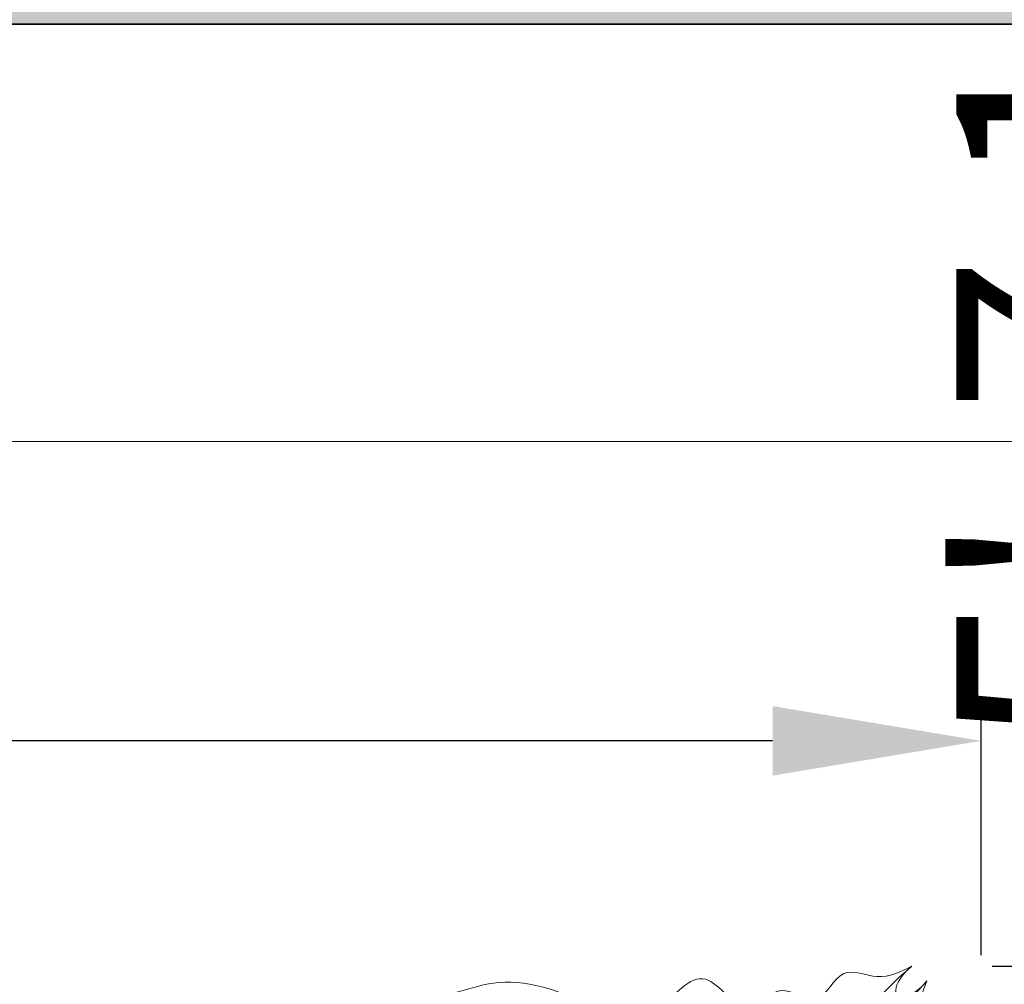
# Model space of a CAD drawing. Units: inches. Extents: x 2083 to 3317, y 1141 to 2115.
# Tile 13 of 256: x 2267 to 2324, y 1361 to 1417. Entities that reach past the tile are written whole.
import ezdxf

# ---------------------------------------------------------------- set-up
doc = ezdxf.new("R2010")
doc.units = ezdxf.units.IN
for name, color, linetype, lineweight in [('A-ANNO-DIMS', 2, 'Continuous', 18), ('A-FLOR-CASE', 8, 'Continuous', 18), ('A-FURN', 8, 'Continuous', 18), ('A-WALL', 7, 'Continuous', 35), ('www.cadblocksfree.com', 7, 'Continuous', 9)]:
    doc.layers.add(name, color=color, linetype=linetype, lineweight=lineweight)
doc.layers.add('A-WALL-PATT', color=251, linetype='Continuous', lineweight=13, true_color=0x636466)
doc.styles.get("Standard").update_dxf_attribs({"font": 'arial.ttf'})
doc.dimstyles.new('ISO-25', dxfattribs={"dimtxt": 12, "dimasz": 12, "dimexe": 1.25, "dimexo": 0.625, "dimtad": 1, "dimlunit": 3, "dimtxsty": 'Standard', "dimcen": 2.5, "dimadec": 0, "dimazin": 0, "dimtfac": 1, "dimtmove": 0, "dimatfit": 3, "dimfxl": 1, "dimarcsym": 0})

# ---------------------------------------------------------------- blocks, each defined once
blk = doc.blocks.new('bed')
at = {"layer": 'www.cadblocksfree.com', "ltscale": 0.2}
for centre, major_axis, ratio, start_param, end_param in [((3429.422, 1388.371), (-3.043, 3.043), 0.168252, 4.250342, 8.316029), ((3430.477, 1387.316), (-1.055, 1.055), 0.453532, 4.422107, 8.144264)]:
    blk.add_ellipse(centre, major_axis=major_axis, ratio=ratio, start_param=start_param, end_param=end_param, dxfattribs=at)
for points, knots in [([(3428.534, 1423.97), (3428.914, 1423.397), (3430.098, 1421.613), (3428.491, 1417.656), (3430.593, 1413.794), (3429.801, 1409.122), (3428.396, 1406.564), (3427.355, 1404.971)], [0, 0, 0, 0, 0.050513, 0.157399, 0.2842023, 0.3628173, 0.5066917, 0.5066917, 0.5066917, 0.5066917]), ([(3431.237, 1387.473), (3430.882, 1388.172), (3430.205, 1389.505), (3431.478, 1391.985), (3428.294, 1393.194), (3430.501, 1395.689), (3427.558, 1397.866), (3431.841, 1400.386), (3426.535, 1404.33), (3426.443, 1408.152), (3426.379, 1410.814)], [0, 0, 0, 0, 2.267059, 4.324559, 6.685584, 8.878641, 11.121502, 14.300359, 17.755284, 25.682856, 25.682856, 25.682856, 25.682856]), ([(3430.32, 1386.556), (3427.327, 1387.653), (3422.148, 1389.55), (3414.529, 1384.137), (3405.607, 1387.046), (3396.29, 1386.314), (3386.838, 1381.282), (3377.742, 1390.272), (3370.778, 1384.799), (3364.626, 1383.966), (3363.275, 1388.265), (3360.778, 1387.151), (3359.446, 1386.556)], [0, 0, 0, 0, 8.93042, 15.449194, 25.485629, 34.878505, 43.598887, 54.554403, 64.16647, 67.461673, 70.610457, 74.213583, 74.213583, 74.213583, 74.213583])]:
    blk.add_open_spline(points, degree=3, knots=knots, dxfattribs=at)
blk = doc.blocks.new('CASEWORK-96X24')
for q in [(0, 0), (24, 96)]:
    blk.add_line((0, 96), q)
blk = doc.blocks.new('*D22')
at = {"layer": 'A-ANNO-DIMS', "color": 0, "lineweight": -2, "transparency": 16777216}
for p, q in [((2235.96, 1362.739), (2235.96, 1376.309)), ((2322.26, 1362.739), (2322.26, 1376.309)), ((2235.96, 1375.059), (2083.007, 1375.059)), ((2310.26, 1375.059), (2247.96, 1375.059))]:
    blk.add_line(p, q, dxfattribs=at)
at = {"layer": 'A-ANNO-DIMS', "color": 0, "transparency": 16777216}
for points in [[(2247.96, 1377.059), (2247.96, 1373.059), (2235.96, 1375.059)], [(2310.26, 1377.059), (2310.26, 1373.059), (2322.26, 1375.059)]]:
    blk.add_solid(points, dxfattribs=at)
at = {"layer": 'Defpoints', "color": 0, "transparency": 16777216}
for p in [(2235.96, 1375.059), (2235.96, 1362.114), (2322.26, 1362.114)]:
    blk.add_point(p, dxfattribs=at)
at = {"layer": 'A-ANNO-DIMS', "color": 0, "transparency": 16777216, "insert": (2153.483, 1381.889), "char_height": 12, "attachment_point": 5}
blk.add_mtext('BED 7\'-2 1/2" TYP.', dxfattribs=at)
blk = doc.blocks.new('*D23')
at = {"layer": 'A-ANNO-DIMS', "color": 0, "lineweight": -2, "transparency": 16777216}
for p, q in [((2335.205, 1362.114), (2335.205, 1476.472)), ((2322.885, 1362.114), (2336.455, 1362.114)), ((2335.205, 1306.473), (2335.205, 1350.114)), ((2322.885, 1294.473), (2336.455, 1294.473))]:
    blk.add_line(p, q, dxfattribs=at)
at = {"layer": 'A-ANNO-DIMS', "color": 0, "transparency": 16777216}
for points in [[(2333.205, 1350.114), (2337.205, 1350.114), (2335.205, 1362.114)], [(2333.205, 1306.473), (2337.205, 1306.473), (2335.205, 1294.473)]]:
    blk.add_solid(points, dxfattribs=at)
at = {"layer": 'Defpoints', "color": 0, "transparency": 16777216}
for p in [(2322.26, 1362.114), (2335.205, 1362.114), (2322.26, 1294.473)]:
    blk.add_point(p, dxfattribs=at)
at = {"layer": 'A-ANNO-DIMS', "color": 0, "transparency": 16777216, "insert": (2328.376, 1425.293), "char_height": 12, "attachment_point": 5, "rotation": 90}
blk.add_mtext('5\'-7 1/2" TYP.', dxfattribs=at)
blk = doc.blocks.new('*D30')
at = {"layer": 'A-ANNO-DIMS', "color": 0, "lineweight": -2, "transparency": 16777216}
for p, q in [((2240.018, 1445.274), (2240.018, 1448.046)), ((2254.329, 1445.274), (2254.329, 1448.046)), ((2228.018, 1446.796), (2216.018, 1446.796)), ((2240.018, 1446.796), (2254.329, 1446.796)), ((2266.329, 1446.796), (2413.765, 1446.796))]:
    blk.add_line(p, q, dxfattribs=at)
at = {"layer": 'A-ANNO-DIMS', "color": 0, "transparency": 16777216}
for points in [[(2228.018, 1448.796), (2228.018, 1444.796), (2240.018, 1446.796)], [(2266.329, 1448.796), (2266.329, 1444.796), (2254.329, 1446.796)]]:
    blk.add_solid(points, dxfattribs=at)
at = {"layer": 'Defpoints', "color": 0, "transparency": 16777216}
for p in [(2254.329, 1446.796), (2240.018, 1444.649), (2254.329, 1444.649)]:
    blk.add_point(p, dxfattribs=at)
at = {"layer": 'A-ANNO-DIMS', "color": 0, "transparency": 16777216, "insert": (2346.047, 1453.625), "char_height": 12, "attachment_point": 5}
blk.add_mtext('WC 1\'-2 1/2" TYP.', dxfattribs=at)

msp = doc.modelspace()

# ---------------------------------------------------------------- hatches: boundary and pattern name
at = {"layer": 'A-WALL-PATT'}
h = msp.add_hatch(color=256, dxfattribs=at)
h.dxf.hatch_style = 1
h.paths.add_polyline_path([(3126.96, 2020.761), (2748.96, 2020.761), (2604.96, 2020.761), (2226.96, 2020.761), (2226.96, 1702.761), (2466.96, 1702.761), (2466.96, 1582.761), (2418.96, 1582.761), (2418.96, 1477.761), (2226.96, 1477.761), (2226.96, 1263.261), (2544.96, 1263.261), (2544.96, 1411.761), (2604.96, 1411.761), (2685.96, 1411.761), (2685.96, 1420.761), (2604.96, 1420.761), (2604.96, 1573.761), (2604.96, 1702.761), (2604.96, 2011.761), (2748.96, 2011.761), (2748.96, 1702.761), (2862.96, 1702.761), (2862.96, 1621.761), (2871.96, 1621.761), (2871.96, 1702.761), (2883.96, 1702.761), (2883.96, 1706.939, -0.026459), (2883.96, 1711.761), (2757.96, 1711.761), (2757.96, 1807.761), (2787.96, 1807.761), (2787.96, 1812.261), (2757.96, 1812.261), (2757.96, 2011.761), (2877.96, 2011.761), (2877.96, 1812.261), (2847.96, 1812.261), (2847.96, 1807.761), (2889.836, 1807.761), (2889.836, 1812.261), (2882.46, 1812.261), (2882.46, 2011.761), (3117.96, 2011.761), (3117.96, 1812.261), (2937.836, 1812.261), (2937.836, 1807.761), (2995.71, 1807.761), (2995.71, 1796.118), (3000.21, 1796.118), (3000.21, 1807.761), (3117.96, 1807.761), (3117.96, 1711.761), (3000.21, 1711.761), (3000.21, 1760.118), (2998.573, 1760.118, -0.020711), (2995.71, 1760.118), (2995.71, 1711.761), (2931.96, 1711.761), (2931.96, 1702.761), (3126.96, 1702.761)])
h.paths.add_polyline_path([(2471.46, 2011.761), (2471.46, 1810.011), (2462.717, 1810.011), (2462.717, 1805.511), (2505.96, 1805.511), (2505.96, 1810.011), (2475.96, 1810.011), (2475.96, 2011.761), (2595.96, 2011.761), (2595.96, 1810.011), (2565.96, 1810.011), (2565.96, 1805.511), (2595.96, 1805.511), (2595.96, 1711.761), (2235.96, 1711.761), (2235.96, 1805.511), (2353.71, 1805.511), (2353.71, 1796.054), (2358.21, 1796.054), (2358.21, 1805.511), (2414.717, 1805.511), (2414.717, 1810.011), (2235.96, 1810.011), (2235.96, 2011.761)], flags=16)
h.paths.add_polyline_path([(2270.205, 1994.61), (2270.205, 1970.61), (2246.205, 1970.61), (2246.205, 1994.61)], flags=0)
edge = h.paths.add_edge_path(flags=0)
edge.add_ellipse((2332.027, 1899.798), major_axis=(-3.043, 3.043), ratio=0.168252, start_angle=-161.3322, end_angle=-156.3071, ccw=False)
edge.add_ellipse((2333.082, 1898.744), major_axis=(-1.055, 1.055), ratio=0.453532, start_angle=-123.371, end_angle=-94.1591)
edge = h.paths.add_edge_path(flags=0)
edge.add_ellipse((2332.027, 1968.876), major_axis=(3.043, 3.043), ratio=0.168252, start_angle=18.6678, end_angle=23.6929)
edge.add_spline(control_points=[(2332.926, 1970.691), (2332.227, 1970.336), (2330.894, 1969.659), (2328.413, 1970.932), (2327.204, 1967.749), (2324.71, 1969.956), (2322.533, 1967.012), (2320.013, 1971.296), (2317.68, 1968.158), (2316.041, 1967.102), (2315.427, 1966.81)], knot_values=[0, 0, 0, 0, 2.267059, 4.324559, 6.685584, 8.878641, 11.121502, 14.300359, 17.755284, 19.732645, 19.732645, 19.732645, 19.732645], degree=3, periodic=0)
edge.add_ellipse((2332.027, 1968.876), major_axis=(3.043, 3.043), ratio=0.168252, start_angle=18.6678, end_angle=23.6929, ccw=False)
edge.add_ellipse((2333.082, 1969.931), major_axis=(1.055, 1.055), ratio=0.453532, start_angle=56.629, end_angle=85.8409, ccw=False)
edge = h.paths.add_edge_path(flags=0)
edge.add_spline(control_points=[(2296.428, 1967.988), (2293.628, 1965.336), (2287.704, 1959.727), (2299.744, 1949.996), (2294.533, 1935.669), (2290.573, 1920.604), (2293.394, 1909.974), (2296.185, 1904.967)], knot_values=[0.099185, 0.099185, 0.099185, 0.099185, 0.345301, 0.619822, 0.982653, 1.386093, 1.810555, 1.810555, 1.810555, 1.810555], degree=3, periodic=0)
edge.add_spline(control_points=[(2296.185, 1904.967), (2297.384, 1902.619), (2298.001, 1901.949), (2298.553, 1901.468)], knot_values=[0.006246, 0.006246, 0.006246, 0.006246, 0.055476, 0.055476, 0.055476, 0.055476], degree=3, periodic=0)
edge.add_spline(control_points=[(2298.553, 1901.468), (2297.259, 1900.923), (2295.225, 1900.232), (2293.06, 1900.614), (2292.101, 1900.788), (2292.09, 1900.791)], knot_values=[0.312835, 0.312835, 0.312835, 0.312835, 0.40178, 0.474987, 0.475903, 0.475903, 0.475903, 0.475903], degree=3, periodic=0)
edge.add_arc((2292.794, 1904.664), 3.937, 215.4209, 259.6982, ccw=False)
edge.add_spline(control_points=[(2289.585, 1902.382), (2289.477, 1902.535), (2289.368, 1902.688), (2289.261, 1902.841)], knot_values=[0.102872, 0.102872, 0.102872, 0.102872, 0.116896, 0.116896, 0.116896, 0.116896], degree=3, periodic=0)
edge.add_spline(control_points=[(2289.261, 1902.841), (2288.687, 1902.55), (2287.64, 1902.02), (2285.881, 1901.874), (2283.853, 1901.504), (2281.72, 1899.711), (2278.467, 1899.493), (2276.157, 1901.883), (2272.259, 1899.804), (2267.778, 1901.843), (2262.244, 1900.184), (2257.415, 1901.782), (2254.318, 1900.726), (2253.178, 1900.337)], knot_values=[0, 0, 0, 0, 1.907977, 3.477176, 5.261074, 7.972851, 11.680248, 13.717921, 16.939592, 22.789562, 27.502503, 33.595215, 37.145618, 37.145618, 37.145618, 37.145618], degree=3, periodic=0)
edge.add_line((2253.178, 1900.337), (2250.244, 1902.841))
edge.add_line((2250.244, 1902.841), (2250.244, 1965.833))
edge.add_line((2250.244, 1965.833), (2253.178, 1968.337))
edge.add_spline(control_points=[(2253.178, 1968.337), (2254.318, 1967.948), (2257.415, 1966.892), (2262.244, 1968.49), (2267.778, 1966.831), (2271.527, 1968.537), (2273.876, 1967.828), (2274.207, 1967.728)], knot_values=[0, 0, 0, 0, 0.09018, 0.244935, 0.364644, 0.513233, 0.537855, 0.537855, 0.537855, 0.537855], degree=3, periodic=0)
edge.add_arc((2274.353, 1963.793), 3.937, 72.0511, 92.1279, ccw=False)
edge.add_arc((2281.297, 1985.23), 18.596, 252.0511, 288.5657)
edge.add_arc((2292.317, 1956.029), 12.646, 71.0268, 113.7782, ccw=False)
edge = h.paths.add_edge_path(flags=0)
edge.add_spline(control_points=[(2274.899, 1951.856), (2275.066, 1951.617), (2275.233, 1951.377), (2275.398, 1951.136)], knot_values=[1.409916, 1.409916, 1.409916, 1.409916, 1.43159, 1.43159, 1.43159, 1.43159], degree=3, periodic=0)
edge.add_spline(control_points=[(2275.398, 1951.136), (2275.792, 1950.562), (2276.179, 1949.984), (2276.546, 1949.397)], knot_values=[1.358238, 1.358238, 1.358238, 1.358238, 1.409916, 1.409916, 1.409916, 1.409916], degree=3, periodic=0)
edge.add_line((2276.546, 1949.397), (2277.437, 1947.862))
edge.add_spline(control_points=[(2277.437, 1947.862), (2276.304, 1945.673), (2274.64, 1942.427), (2274.632, 1938.094), (2272.799, 1930.852), (2274.356, 1943.897), (2275.948, 1947.923), (2276.546, 1949.397)], knot_values=[0.005632, 0.005632, 0.005632, 0.005632, 0.186014, 0.266002, 0.357087, 0.59639, 0.739732, 0.739732, 0.739732, 0.739732], degree=3, periodic=0)
edge.add_spline(control_points=[(2276.546, 1949.397), (2276.179, 1949.984), (2275.792, 1950.562), (2275.398, 1951.136)], knot_values=[1.358238, 1.358238, 1.358238, 1.358238, 1.409916, 1.409916, 1.409916, 1.409916], degree=3, periodic=0)
edge.add_spline(control_points=[(2275.398, 1951.136), (2274.943, 1950.08), (2274.208, 1948.025), (2273.935, 1944.851), (2272.469, 1937.627), (2273.466, 1945.696), (2274.701, 1951.059), (2274.899, 1951.856)], knot_values=[0.104364, 0.104364, 0.104364, 0.104364, 0.189636, 0.269624, 0.36071, 0.600013, 0.644622, 0.644622, 0.644622, 0.644622], degree=3, periodic=0)
h.paths.add_polyline_path([(2269.168, 1963.128, -0.357527), (2268.171, 1960.976, -0.092561), (2268.171, 1939.436, -0.357527), (2269.168, 1937.285, -0.357527), (2267.016, 1938.282, -0.164785), (2254.686, 1938.282, -0.357527), (2252.534, 1937.285, -0.357527), (2253.531, 1939.436, -0.092561), (2253.531, 1960.976, -0.357527), (2252.534, 1963.128, -0.357527), (2254.686, 1962.131, -0.164785), (2267.016, 1962.131, -0.357527)], flags=0)
h.paths.add_polyline_path([(2248.874, 1967.802), (2248.874, 1957.028), (2249.458, 1957.028), (2249.458, 1911.647), (2248.874, 1911.647), (2248.874, 1900.873), (2246.512, 1900.873, 0.197327), (2244.15, 1902.457), (2244.15, 1966.218, 0.197327), (2246.512, 1967.802)], flags=0)
h.paths.add_polyline_path([(2269.168, 1931.389, -0.357527), (2268.171, 1929.238, -0.092561), (2268.171, 1907.698, -0.357527), (2269.168, 1905.547, -0.357527), (2267.016, 1906.544, -0.164785), (2254.686, 1906.544, -0.357527), (2252.534, 1905.547, -0.357527), (2253.531, 1907.698, -0.092561), (2253.531, 1929.238, -0.357527), (2252.534, 1931.389, -0.357527), (2254.686, 1930.392, -0.164785), (2267.016, 1930.392, -0.357527)], flags=0)
edge = h.paths.add_edge_path(flags=0)
edge.add_spline(control_points=[(2276.197, 1906.724), (2276.168, 1909.029), (2276.114, 1913.372), (2270.598, 1924.925), (2273.905, 1919.013), (2275.922, 1916.262), (2275.475, 1912.402), (2277.258, 1910.381), (2276.696, 1908.225), (2276.646, 1906.813), (2276.618, 1906.008)], knot_values=[0, 0, 0, 0, 8.61026, 16.221274, 18.843057, 23.804898, 27.440828, 29.356102, 31.203478, 33.650687, 33.650687, 33.650687, 33.650687], degree=3, periodic=0)
edge.add_spline(control_points=[(2276.618, 1906.008), (2276.623, 1905.624), (2276.498, 1904.629), (2275.442, 1903.855), (2274.937, 1903.08), (2274.859, 1902.841)], knot_values=[0.156488, 0.156488, 0.156488, 0.156488, 0.184398, 0.231376, 0.250598, 0.250598, 0.250598, 0.250598], degree=3, periodic=0)
edge.add_line((2274.859, 1902.841), (2276.506, 1902.841))
edge.add_spline(control_points=[(2276.506, 1902.841), (2276.788, 1903.085), (2277.665, 1904.125), (2278.25, 1904.341), (2277.654, 1908.527), (2278.156, 1906.228), (2278.1, 1905.286), (2278.847, 1904.069), (2277.857, 1903.415), (2277.874, 1902.991), (2277.904, 1902.841)], knot_values=[0.059574, 0.059574, 0.059574, 0.059574, 0.080753, 0.103741, 0.16972, 0.176036, 0.207137, 0.240474, 0.262341, 0.27366, 0.27366, 0.27366, 0.27366], degree=3, periodic=0)
edge.add_line((2277.904, 1902.841), (2280.03, 1902.841))
edge.add_spline(control_points=[(2280.03, 1902.841), (2279.888, 1903.088), (2279.499, 1903.982), (2280.152, 1905.939), (2278.104, 1909.658), (2279.762, 1907.185), (2280.328, 1904.875), (2280.485, 1903.49), (2281.463, 1903.249), (2281.758, 1902.936), (2281.834, 1902.841)], knot_values=[0.013856, 0.013856, 0.013856, 0.013856, 0.034874, 0.088867, 0.107879, 0.126738, 0.158714, 0.193757, 0.217487, 0.226722, 0.226722, 0.226722, 0.226722], degree=3, periodic=0)
edge.add_spline(control_points=[(2281.834, 1902.841), (2281.788, 1902.827), (2281.647, 1902.783), (2281.396, 1902.859), (2281.088, 1902.985), (2280.721, 1903.061), (2280.333, 1903.026), (2280.125, 1902.899), (2280.03, 1902.841)], knot_values=[0, 0, 0, 0, 0.14413, 0.435517, 0.749276, 1.153046, 1.548371, 1.878348, 1.878348, 1.878348, 1.878348], degree=3, periodic=0)
edge.add_line((2280.03, 1902.841), (2277.904, 1902.841))
edge.add_spline(control_points=[(2277.904, 1902.841), (2277.893, 1902.796), (2277.865, 1902.68), (2277.607, 1902.687), (2277.274, 1902.801), (2276.838, 1902.62), (2276.584, 1902.789), (2276.506, 1902.841)], knot_values=[0, 0, 0, 0, 0.127189, 0.326199, 0.628009, 1.24357, 1.515331, 1.515331, 1.515331, 1.515331], degree=3, periodic=0)
edge.add_line((2276.506, 1902.841), (2274.859, 1902.841))
edge.add_spline(control_points=[(2274.859, 1902.841), (2274.814, 1902.899), (2274.725, 1903.013), (2274.493, 1903.119), (2274.244, 1902.961), (2273.937, 1903.185), (2273.614, 1902.983), (2273.408, 1902.883), (2273.322, 1902.841)], knot_values=[0, 0, 0, 0, 0.21843, 0.436957, 0.687977, 0.990379, 1.398396, 1.69185, 1.69185, 1.69185, 1.69185], degree=3, periodic=0)
edge.add_spline(control_points=[(2273.322, 1902.841), (2273.617, 1903.446), (2274.274, 1904.538), (2276.027, 1904.574), (2276.207, 1906.584), (2276.197, 1906.724)], knot_values=[0.012227, 0.012227, 0.012227, 0.012227, 0.059472, 0.106218, 0.134458, 0.134458, 0.134458, 0.134458], degree=3, periodic=0)
h.paths.add_polyline_path([(2270.776, 1897.79), (2270.776, 1873.79), (2246.776, 1873.79), (2246.776, 1897.79)], flags=0)
h.paths.add_polyline_path([(2353.71, 1760.005), (2353.71, 1760.054), (2358.21, 1760.054, -0.033729)], flags=0)
h.paths.add_polyline_path([(2321.819, 1737.529), (2341.995, 1737.529, -0.414214), (2343.203, 1736.321), (2343.203, 1721.021, -0.414214), (2341.995, 1719.813), (2321.819, 1719.813, -0.414214), (2320.611, 1721.021), (2320.611, 1736.321, -0.414214)], flags=0)
h.paths.add_polyline_path([(2324.235, 1736.321), (2339.579, 1736.321, -0.414214), (2341.995, 1733.905), (2341.995, 1725.45, -0.414214), (2339.579, 1723.034), (2333.681, 1723.034), (2333.845, 1722.045, -0.870646), (2335.425, 1721.826, -0.767327), (2333.923, 1721.423), (2331.291, 1721.423, -0.767327), (2329.788, 1721.826, -0.870646), (2331.368, 1722.045), (2331.533, 1723.034), (2324.235, 1723.034, -0.414214), (2321.819, 1725.45), (2321.819, 1733.905, -0.414214)], flags=0)
h.paths.add_polyline_path([(2570.484, 1928.615), (2589.684, 1928.615), (2590.169, 1928.615), (2590.169, 1904.993), (2570.484, 1904.993)], flags=0)
h.paths.add_polyline_path([(2574.447, 1927.264, -1), (2572.829, 1927.264, -1)], flags=0)
h.paths.add_polyline_path([(2573.09, 1926.941), (2573.925, 1927.776), (2574.148, 1927.553), (2573.313, 1926.718)], flags=0)
h.paths.add_polyline_path([(2578.779, 1919.73, -1), (2571.592, 1919.73, -1)], flags=0)
h.paths.add_polyline_path([(2578.385, 1919.73, -1), (2571.985, 1919.73, -1)], flags=0)
h.paths.add_polyline_path([(2331.596, 1729.476, -1), (2333.618, 1729.476, -1)], flags=0)
h.paths.add_polyline_path([(2578.034, 1927.264, -1), (2576.416, 1927.264, -1)], flags=0)
h.paths.add_polyline_path([(2576.689, 1927.531), (2576.912, 1927.754), (2577.747, 1926.919), (2577.524, 1926.696)], flags=0)
h.paths.add_polyline_path([(2578.139, 1909.86, -1), (2572.232, 1909.86, -1)], flags=0)
h.paths.add_polyline_path([(2577.745, 1909.86, -1), (2572.625, 1909.86, -1)], flags=0)
h.paths.add_polyline_path([(2583.798, 1927.264, -1), (2582.179, 1927.264, -1)], flags=0)
h.paths.add_polyline_path([(2582.719, 1927.754), (2583.554, 1926.919), (2583.331, 1926.696), (2582.496, 1927.531)], flags=0)
h.paths.add_polyline_path([(2582.496, 1927.531), (2582.719, 1927.754), (2583.554, 1926.919), (2583.331, 1926.696)], flags=0)
h.paths.add_polyline_path([(2587.739, 1920.53, -1), (2581.832, 1920.53, -1)], flags=0)
h.paths.add_polyline_path([(2587.345, 1920.53, -1), (2582.225, 1920.53, -1)], flags=0)
h.paths.add_polyline_path([(2587.385, 1927.264, -1), (2585.766, 1927.264, -1)], flags=0)
h.paths.add_polyline_path([(2586.082, 1926.98), (2586.917, 1927.815), (2587.14, 1927.593), (2586.305, 1926.758)], flags=0)
h.paths.add_polyline_path([(2588.379, 1910.66, -1), (2581.192, 1910.66, -1)], flags=0)
h.paths.add_polyline_path([(2587.985, 1910.66, -1), (2581.585, 1910.66, -1)], flags=0)
h.paths.add_polyline_path([(2417.168, 1729.478), (2437.344, 1729.478, -0.414214), (2438.552, 1728.27), (2438.552, 1712.969, -0.414214), (2437.344, 1711.761), (2417.168, 1711.761, -0.414214), (2415.96, 1712.969), (2415.96, 1728.27, -0.414214)], flags=0)
h.paths.add_polyline_path([(2419.584, 1728.27), (2434.928, 1728.27, -0.414214), (2437.344, 1725.854), (2437.344, 1717.398, -0.414214), (2434.928, 1714.983), (2429.029, 1714.983), (2429.194, 1713.994, -0.870646), (2430.774, 1713.775, -0.767327), (2429.271, 1713.372), (2426.64, 1713.372, -0.767327), (2425.137, 1713.775, -0.870646), (2426.717, 1713.994), (2426.882, 1714.983), (2419.584, 1714.983, -0.414214), (2417.168, 1717.398), (2417.168, 1725.854, -0.414214)], flags=0)
h.paths.add_polyline_path([(2419.584, 1728.27), (2434.928, 1728.27, -0.414214), (2437.344, 1725.854), (2437.344, 1717.398, -0.414214), (2434.928, 1714.983), (2429.029, 1714.983), (2428.358, 1719.009), (2427.553, 1719.009), (2426.882, 1714.983), (2419.584, 1714.983, -0.414214), (2417.168, 1717.398), (2417.168, 1725.854, -0.414214)], flags=0)
h.paths.add_polyline_path([(2426.944, 1721.425, -1), (2428.967, 1721.425, -1)], flags=0)
h.paths.add_polyline_path([(2475.96, 1702.761), (2595.96, 1702.761), (2595.96, 1582.761), (2475.96, 1582.761)], flags=16)
h.paths.add_polyline_path([(2427.96, 1573.761), (2595.96, 1573.761), (2595.96, 1468.761), (2595.96, 1420.761), (2384.46, 1420.761), (2384.46, 1468.761), (2427.96, 1468.761)], flags=16)
h.paths.add_polyline_path([(2379.96, 1468.761), (2379.96, 1420.761), (2235.96, 1420.761), (2235.96, 1468.761)], flags=16)
h.paths.add_polyline_path([(2317.816, 1466.696), (2337.992, 1466.696, -0.414214), (2339.2, 1465.488), (2339.2, 1450.187, -0.414214), (2337.992, 1448.979), (2317.816, 1448.979, -0.414214), (2316.608, 1450.187), (2316.608, 1465.488, -0.414214)], flags=0)
h.paths.add_polyline_path([(2320.232, 1465.488), (2335.576, 1465.488, -0.414214), (2337.992, 1463.072), (2337.992, 1454.616, -0.414214), (2335.576, 1452.2), (2329.677, 1452.2), (2329.842, 1451.212, -0.870646), (2331.422, 1450.992, -0.767327), (2329.92, 1450.59), (2327.288, 1450.59, -0.767327), (2325.785, 1450.992, -0.870646), (2327.365, 1451.212), (2327.53, 1452.2), (2320.232, 1452.2, -0.414214), (2317.816, 1454.616), (2317.816, 1463.072, -0.414214)], flags=0)
h.paths.add_polyline_path([(2320.232, 1465.488), (2335.576, 1465.488, -0.414214), (2337.992, 1463.072), (2337.992, 1454.616, -0.414214), (2335.576, 1452.2), (2329.677, 1452.2), (2329.006, 1456.227), (2328.201, 1456.227), (2327.53, 1452.2), (2320.232, 1452.2, -0.414214), (2317.816, 1454.616), (2317.816, 1463.072, -0.414214)], flags=0)
h.paths.add_polyline_path([(2327.593, 1458.643, -1), (2329.615, 1458.643, -1)], flags=0)
h.paths.add_polyline_path([(2244.412, 1433.34), (2241.921, 1433.34, -0.414214), (2240.018, 1435.244), (2240.018, 1440.953, -0.414211), (2241.921, 1442.856), (2244.412, 1442.856, -1.976472)], flags=0)
h.paths.add_polyline_path([(2245.357, 1434.398, -0.414214), (2245.357, 1441.799, -2.144098)], flags=0)
h.paths.add_polyline_path([(2535.96, 1416.261), (2535.96, 1272.261), (2235.96, 1272.261), (2235.96, 1416.261)], flags=16)
h.paths.add_polyline_path([(2260.12, 1384.293), (2260.12, 1362.039), (2237.865, 1362.039), (2237.865, 1384.293)], flags=0)
edge = h.paths.add_edge_path(flags=0)
edge.add_line((2318.252, 1362.093), (2318.146, 1362.001))
edge.add_ellipse((2317.445, 1360.431), major_axis=(2.822, 2.822), ratio=0.168252, start_angle=18.6678, end_angle=20.9481, ccw=False)
edge.add_ellipse((2318.423, 1361.409), major_axis=(0.978, 0.978), ratio=0.453532, start_angle=56.629, end_angle=70.2262, ccw=False)
edge = h.paths.add_edge_path(flags=0)
edge.add_line((2319.107, 1295.571), (2319.015, 1295.677))
edge.add_ellipse((2317.445, 1296.378), major_axis=(-2.822, 2.822), ratio=0.168252, start_angle=-161.3322, end_angle=-159.0519, ccw=False)
edge.add_ellipse((2318.423, 1295.4), major_axis=(-0.978, 0.978), ratio=0.453532, start_angle=-123.371, end_angle=-109.7738)
edge = h.paths.add_edge_path(flags=0)
edge.add_spline(control_points=[(2284.21, 1301.17), (2284.581, 1300.445), (2284.891, 1299.892), (2285.16, 1299.461)], knot_values=[0.039066, 0.039066, 0.039066, 0.039066, 0.055476, 0.055476, 0.055476, 0.055476], degree=3, periodic=0)
edge.add_line((2285.16, 1299.461), (2284.21, 1301.17))
edge = h.paths.add_edge_path(flags=0)
edge.add_line((2280.412, 1297.298), (2283.37, 1297.036))
edge.add_line((2283.37, 1297.036), (2286.406, 1297.926))
edge.add_spline(control_points=[(2286.406, 1297.926), (2285.305, 1297.463), (2284.345, 1297.129), (2283.37, 1297.036)], knot_values=[0.394369, 0.394369, 0.394369, 0.394369, 0.475903, 0.475903, 0.475903, 0.475903], degree=3, periodic=0)
edge.add_spline(control_points=[(2283.37, 1297.036), (2283.281, 1297.028), (2282.316, 1296.957), (2281.313, 1297.134), (2280.423, 1297.296), (2280.412, 1297.298)], knot_values=[0.312835, 0.312835, 0.312835, 0.312835, 0.320246, 0.393453, 0.394369, 0.394369, 0.394369, 0.394369], degree=3, periodic=0)
edge = h.paths.add_edge_path(flags=0)
edge.add_line((2284.436, 1359.607), (2280.446, 1355.328))
edge.add_line((2280.446, 1355.328), (2279.58, 1351.018))
edge.add_line((2279.58, 1351.018), (2282.413, 1346.58))
edge.add_spline(control_points=[(2282.413, 1346.58), (2283.153, 1345.589), (2284.253, 1344.029), (2284.801, 1342.387), (2284.935, 1341.806)], knot_values=[1.240098, 1.240098, 1.240098, 1.240098, 1.332892, 1.382712, 1.382712, 1.382712, 1.382712], degree=3, periodic=0)
edge.add_spline(control_points=[(2284.935, 1341.806), (2285.319, 1340.141), (2285.233, 1338.409), (2284.91, 1336.654)], knot_values=[1.097484, 1.097484, 1.097484, 1.097484, 1.240098, 1.240098, 1.240098, 1.240098], degree=3, periodic=0)
edge.add_spline(control_points=[(2284.91, 1336.654), (2284.587, 1334.899), (2284.027, 1333.12), (2283.463, 1331.361)], knot_values=[0.95487, 0.95487, 0.95487, 0.95487, 1.097484, 1.097484, 1.097484, 1.097484], degree=3, periodic=0)
edge.add_line((2283.463, 1331.361), (2281.89, 1326.153))
edge.add_line((2281.89, 1326.153), (2280.756, 1321.056))
edge.add_line((2280.756, 1321.056), (2280.299, 1316.002))
edge.add_line((2280.299, 1316.002), (2280.716, 1310.95))
edge.add_line((2280.716, 1310.95), (2282.028, 1305.972))
edge.add_line((2282.028, 1305.972), (2284.21, 1301.17))
edge.add_spline(control_points=[(2284.21, 1301.17), (2283.341, 1302.73), (2282.612, 1304.336), (2282.028, 1305.972)], knot_values=[0.099185, 0.099185, 0.099185, 0.099185, 0.241799, 0.241799, 0.241799, 0.241799], degree=3, periodic=0)
edge.add_spline(control_points=[(2282.028, 1305.972), (2281.444, 1307.608), (2281.005, 1309.273), (2280.716, 1310.95)], knot_values=[0.241799, 0.241799, 0.241799, 0.241799, 0.384413, 0.384413, 0.384413, 0.384413], degree=3, periodic=0)
edge.add_spline(control_points=[(2280.716, 1310.95), (2280.433, 1312.588), (2280.289, 1314.277), (2280.299, 1315.962), (2280.299, 1316.002)], knot_values=[0.384413, 0.384413, 0.384413, 0.384413, 0.523647, 0.527028, 0.527028, 0.527028, 0.527028], degree=3, periodic=0)
edge.add_spline(control_points=[(2280.299, 1316.002), (2280.312, 1317.687), (2280.478, 1319.368), (2280.756, 1321.056)], knot_values=[0.527028, 0.527028, 0.527028, 0.527028, 0.669642, 0.669642, 0.669642, 0.669642], degree=3, periodic=0)
edge.add_spline(control_points=[(2280.756, 1321.056), (2281.035, 1322.744), (2281.426, 1324.44), (2281.89, 1326.153)], knot_values=[0.669642, 0.669642, 0.669642, 0.669642, 0.812256, 0.812256, 0.812256, 0.812256], degree=3, periodic=0)
edge.add_spline(control_points=[(2281.89, 1326.153), (2282.264, 1327.533), (2282.788, 1329.262), (2283.353, 1331.018), (2283.463, 1331.361)], knot_values=[0.812256, 0.812256, 0.812256, 0.812256, 0.927087, 0.95487, 0.95487, 0.95487, 0.95487], degree=3, periodic=0)
edge.add_line((2283.463, 1331.361), (2284.91, 1336.654))
edge.add_line((2284.91, 1336.654), (2284.935, 1341.806))
edge.add_line((2284.935, 1341.806), (2282.413, 1346.58))
edge.add_spline(control_points=[(2282.413, 1346.58), (2281.275, 1348.104), (2280.078, 1349.57), (2279.58, 1351.018)], knot_values=[1.382712, 1.382712, 1.382712, 1.382712, 1.525326, 1.525326, 1.525326, 1.525326], degree=3, periodic=0)
edge.add_spline(control_points=[(2279.58, 1351.018), (2279.443, 1351.415), (2279.136, 1352.857), (2279.735, 1354.29), (2280.446, 1355.328)], knot_values=[1.525326, 1.525326, 1.525326, 1.525326, 1.564439, 1.667941, 1.667941, 1.667941, 1.667941], degree=3, periodic=0)
edge.add_spline(control_points=[(2280.446, 1355.328), (2281.426, 1356.758), (2282.931, 1358.183), (2284.436, 1359.607)], knot_values=[1.667941, 1.667941, 1.667941, 1.667941, 1.810555, 1.810555, 1.810555, 1.810555], degree=3, periodic=0)
edge.add_arc((2280.623, 1348.518), 11.726, 71.0268, 113.7782)
edge.add_arc((2270.405, 1375.595), 17.244, 252.0511, 288.5657, ccw=False)
edge.add_arc((2263.966, 1355.718), 3.651, 72.0511, 92.1279)
edge.add_arc((2263.966, 1355.718), 3.651, 92.1279, 177.9851)
edge.add_spline(control_points=[(2260.318, 1355.846), (2260.26, 1354.221), (2260.551, 1350.187), (2262.999, 1346.766), (2264.473, 1344.649)], knot_values=[1.43159, 1.43159, 1.43159, 1.43159, 1.564144, 1.770695, 1.770695, 1.770695, 1.770695], degree=3, periodic=0)
edge.add_line((2264.473, 1344.649), (2264.936, 1343.983))
edge.add_spline(control_points=[(2263.801, 1340.248), (2263.843, 1340.514), (2264.067, 1341.756), (2264.513, 1343.002), (2264.935, 1343.981)], knot_values=[0.53657, 0.53657, 0.53657, 0.53657, 0.559349, 0.644622, 0.644622, 0.644622, 0.644622], degree=3, periodic=0)
edge.add_spline(control_points=[(2264.935, 1343.981), (2265.118, 1343.715), (2265.299, 1343.448), (2265.477, 1343.179)], knot_values=[1.384077, 1.384077, 1.384077, 1.384077, 1.409916, 1.409916, 1.409916, 1.409916], degree=3, periodic=0)
edge.add_spline(control_points=[(2265.477, 1343.179), (2265.655, 1342.911), (2265.829, 1342.641), (2265.999, 1342.369)], knot_values=[1.358238, 1.358238, 1.358238, 1.358238, 1.384077, 1.384077, 1.384077, 1.384077], degree=3, periodic=0)
edge.add_line((2265.999, 1342.369), (2266.826, 1340.946))
edge.add_spline(control_points=[(2266.826, 1340.946), (2268.894, 1337.09), (2271.398, 1325.843), (2270.516, 1310.569), (2275.919, 1301.861), (2277.79, 1299.199)], knot_values=[0.116896, 0.116896, 0.116896, 0.116896, 0.472987, 1.050969, 1.313793, 1.313793, 1.313793, 1.313793], degree=3, periodic=0)
edge.add_spline(control_points=[(2277.79, 1299.199), (2277.839, 1299.128), (2277.889, 1299.057), (2277.94, 1298.987)], knot_values=[0.109884, 0.109884, 0.109884, 0.109884, 0.116896, 0.116896, 0.116896, 0.116896], degree=3, periodic=0)
edge.add_line((2277.94, 1298.987), (2277.789, 1299.199))
edge.add_spline(control_points=[(2277.789, 1299.199), (2277.257, 1298.929), (2276.286, 1298.438), (2275.039, 1298.334), (2274.383, 1298.239), (2274.215, 1298.209)], knot_values=[33.12187, 33.12187, 33.12187, 33.12187, 35.029056, 36.598255, 37.144827, 37.144827, 37.144827, 37.144827], degree=3, periodic=0)
edge.add_line((2274.215, 1298.209), (2273.073, 1297.893))
edge.add_spline(control_points=[(2273.073, 1297.893), (2272.323, 1297.58), (2271.039, 1296.511), (2269.248, 1296.226), (2268.423, 1296.375)], knot_values=[26.532584, 26.532584, 26.532584, 26.532584, 29.198919, 31.839101, 31.839101, 31.839101, 31.839101], degree=3, periodic=0)
edge.add_line((2268.423, 1296.375), (2263.879, 1297.458))
edge.add_spline(control_points=[(2263.879, 1297.458), (2263.556, 1297.359), (2261.86, 1296.839), (2260.239, 1297.282), (2258.933, 1297.516)], knot_values=[15.919551, 15.919551, 15.919551, 15.919551, 16.939592, 21.226067, 21.226067, 21.226067, 21.226067], degree=3, periodic=0)
edge.add_line((2258.933, 1297.516), (2254.055, 1297.329))
edge.add_spline(control_points=[(2254.055, 1297.329), (2253.756, 1297.296), (2252.114, 1297.165), (2250.462, 1297.544), (2249.13, 1297.668)], knot_values=[5.306517, 5.306517, 5.306517, 5.306517, 6.276435, 10.613034, 10.613034, 10.613034, 10.613034], degree=3, periodic=0)
edge.add_line((2249.13, 1297.668), (2244.332, 1296.878))
edge.add_line((2244.332, 1296.878), (2241.611, 1299.199))
edge.add_line((2241.611, 1299.199), (2241.611, 1357.609))
edge.add_line((2241.611, 1357.609), (2244.332, 1359.931))
edge.add_line((2244.332, 1359.931), (2252.729, 1359.543))
edge.add_spline(control_points=[(2252.729, 1359.543), (2252.871, 1359.546), (2253.306, 1359.548), (2253.74, 1359.514), (2254.032, 1359.482)], knot_values=[0.233291, 0.233291, 0.233291, 0.233291, 0.244935, 0.268927, 0.268927, 0.268927, 0.268927], degree=3, periodic=0)
edge.add_line((2254.032, 1359.482), (2259.587, 1359.416))
edge.add_spline(control_points=[(2259.587, 1359.416), (2260.677, 1359.629), (2262.073, 1359.897), (2263.524, 1359.459), (2263.83, 1359.366)], knot_values=[0.422516, 0.422516, 0.422516, 0.422516, 0.513233, 0.537855, 0.537855, 0.537855, 0.537855], degree=3, periodic=0)
edge.add_arc((2263.966, 1355.718), 3.651, 72.0511, 92.1279, ccw=False)
edge.add_arc((2270.405, 1375.595), 17.244, 252.0511, 288.5657)
edge.add_arc((2280.623, 1348.518), 11.726, 71.0268, 113.7782, ccw=False)
h.paths.add_polyline_path([(2240.341, 1359.435), (2240.341, 1349.444), (2240.882, 1349.444), (2240.882, 1307.365), (2240.341, 1307.365), (2240.341, 1297.374), (2238.15, 1297.374, 0.197327), (2235.96, 1298.843), (2235.96, 1357.966, 0.197327), (2238.15, 1359.435)], flags=0)
h.paths.add_polyline_path([(2259.158, 1355.101, -0.357527), (2258.233, 1353.106, -0.092561), (2258.233, 1333.133, -0.357527), (2259.158, 1331.138, -0.357527), (2257.163, 1332.062, -0.164785), (2245.729, 1332.062, -0.357527), (2243.735, 1331.138, -0.357527), (2244.659, 1333.133, -0.092561), (2244.659, 1353.106, -0.357527), (2243.735, 1355.101, -0.357527), (2245.729, 1354.176, -0.164785), (2257.163, 1354.176, -0.357527)], flags=0)
edge = h.paths.add_edge_path(flags=0)
edge.add_line((2265.999, 1342.369), (2266.826, 1340.946))
edge.add_line((2266.826, 1340.946), (2265.308, 1337.814))
edge.add_line((2265.308, 1337.814), (2264.358, 1334.653))
edge.add_line((2264.358, 1334.653), (2264.262, 1333.8))
edge.add_spline(control_points=[(2264.262, 1333.8), (2264.208, 1333.187), (2264.162, 1332.366), (2264.007, 1331.414), (2263.969, 1331.202)], knot_values=[0.464444, 0.464444, 0.464444, 0.464444, 0.516691, 0.531608, 0.531608, 0.531608, 0.531608], degree=3, periodic=0)
edge.add_spline(control_points=[(2263.969, 1331.202), (2263.775, 1330.119), (2263.424, 1328.791), (2263.257, 1328.531), (2263.234, 1328.515)], knot_values=[0.372682, 0.372682, 0.372682, 0.372682, 0.44885, 0.464444, 0.464444, 0.464444, 0.464444], degree=3, periodic=0)
edge.add_spline(control_points=[(2263.234, 1328.515), (2263.096, 1328.42), (2263.131, 1329.301), (2263.275, 1330.616)], knot_values=[0.280919, 0.280919, 0.280919, 0.280919, 0.372682, 0.372682, 0.372682, 0.372682], degree=3, periodic=0)
edge.add_spline(control_points=[(2263.275, 1330.616), (2263.419, 1331.93), (2263.672, 1333.677), (2263.97, 1335.315)], knot_values=[0.189157, 0.189157, 0.189157, 0.189157, 0.280919, 0.280919, 0.280919, 0.280919], degree=3, periodic=0)
edge.add_spline(control_points=[(2263.97, 1335.315), (2264.1, 1336.032), (2264.419, 1337.622), (2264.755, 1338.864), (2264.947, 1339.491)], knot_values=[0.097394, 0.097394, 0.097394, 0.097394, 0.137578, 0.189157, 0.189157, 0.189157, 0.189157], degree=3, periodic=0)
edge.add_spline(control_points=[(2264.947, 1339.491), (2265.29, 1340.606), (2265.644, 1341.494), (2265.999, 1342.369)], knot_values=[0.005632, 0.005632, 0.005632, 0.005632, 0.097394, 0.097394, 0.097394, 0.097394], degree=3, periodic=0)
h.paths.add_polyline_path([(2259.158, 1325.671, -0.357527), (2258.233, 1323.676, -0.092561), (2258.233, 1303.703, -0.357527), (2259.158, 1301.708, -0.357527), (2257.163, 1302.633, -0.164785), (2245.729, 1302.633, -0.357527), (2243.735, 1301.708, -0.357527), (2244.659, 1303.703, -0.092561), (2244.659, 1323.676, -0.357527), (2243.735, 1325.671, -0.357527), (2245.729, 1324.747, -0.164785), (2257.163, 1324.747, -0.357527)], flags=0)
edge = h.paths.add_edge_path(flags=0)
edge.add_spline(control_points=[(2261.709, 1317.311), (2261.679, 1317.418), (2261.762, 1317.389), (2262.491, 1316.09), (2262.962, 1315.301)], knot_values=[14.955861, 14.955861, 14.955861, 14.955861, 16.221274, 18.694826, 18.694826, 18.694826, 18.694826], degree=3, periodic=0)
edge.add_spline(control_points=[(2262.962, 1315.301), (2262.99, 1315.254), (2263.702, 1314.067), (2264.349, 1313.127), (2264.73, 1312.164)], knot_values=[18.694826, 18.694826, 18.694826, 18.694826, 18.843057, 22.433791, 22.433791, 22.433791, 22.433791], degree=3, periodic=0)
edge.add_spline(control_points=[(2264.73, 1312.164), (2264.876, 1311.796), (2265.177, 1310.77), (2265.143, 1309.559), (2265.248, 1308.824)], knot_values=[22.433791, 22.433791, 22.433791, 22.433791, 23.804898, 26.172756, 26.172756, 26.172756, 26.172756], degree=3, periodic=0)
edge.add_line((2265.248, 1308.824), (2265.851, 1307.172))
edge.add_spline(control_points=[(2265.851, 1307.172), (2266.065, 1306.822), (2266.384, 1306.332), (2266.424, 1305.781), (2266.42, 1305.611)], knot_values=[28.062562, 28.062562, 28.062562, 28.062562, 29.356102, 29.911721, 29.911721, 29.911721, 29.911721], degree=3, periodic=0)
edge.add_spline(control_points=[(2266.42, 1305.611), (2266.416, 1305.433), (2266.394, 1305.25), (2266.365, 1305.066)], knot_values=[29.911721, 29.911721, 29.911721, 29.911721, 30.497837, 30.497837, 30.497837, 30.497837], degree=3, periodic=0)
edge.add_line((2266.365, 1305.066), (2266.066, 1302.136))
edge.add_spline(control_points=[(2266.066, 1302.136), (2266.071, 1301.78), (2265.998, 1301.2), (2265.663, 1300.759), (2265.509, 1300.586)], knot_values=[0.156488, 0.156488, 0.156488, 0.156488, 0.184398, 0.203543, 0.203543, 0.203543, 0.203543], degree=3, periodic=0)
edge.add_line((2265.509, 1300.586), (2264.435, 1299.199))
edge.add_line((2264.435, 1299.199), (2265.962, 1299.199))
edge.add_line((2265.962, 1299.199), (2267.336, 1301.175))
edge.add_line((2267.336, 1301.175), (2267.312, 1301.986))
edge.add_spline(control_points=[(2267.312, 1301.986), (2267.261, 1302.862), (2267.16, 1303.737), (2267.271, 1303.326)], knot_values=[0.126229, 0.126229, 0.126229, 0.126229, 0.166617, 0.166617, 0.166617, 0.166617], degree=3, periodic=0)
edge.add_spline(control_points=[(2267.271, 1303.326), (2267.28, 1303.294), (2267.31, 1303.175), (2267.373, 1302.884), (2267.406, 1302.683), (2267.418, 1302.601)], knot_values=[0.166617, 0.166617, 0.166617, 0.166617, 0.16972, 0.176036, 0.180765, 0.180765, 0.180765, 0.180765], degree=3, periodic=0)
edge.add_spline(control_points=[(2267.744, 1300.988), (2267.688, 1301.151), (2267.481, 1301.657), (2267.484, 1302.145), (2267.418, 1302.601)], knot_values=[0.180765, 0.180765, 0.180765, 0.180765, 0.193767, 0.220139, 0.220139, 0.220139, 0.220139], degree=3, periodic=0)
edge.add_line((2267.418, 1302.601), (2267.744, 1300.988))
edge.add_spline(control_points=[(2267.744, 1300.988), (2267.832, 1300.732), (2267.932, 1300.31), (2267.555, 1299.975), (2267.429, 1299.829)], knot_values=[0.220139, 0.220139, 0.220139, 0.220139, 0.240474, 0.25489, 0.25489, 0.25489, 0.25489], degree=3, periodic=0)
edge.add_line((2267.429, 1299.829), (2267.258, 1299.199))
edge.add_line((2267.258, 1299.199), (2269.23, 1299.199))
edge.add_spline(control_points=[(2269.23, 1299.199), (2269.099, 1299.429), (2268.843, 1300.016), (2269.012, 1300.916), (2268.947, 1301.661)], knot_values=[0.013856, 0.013856, 0.013856, 0.013856, 0.034874, 0.067073, 0.067073, 0.067073, 0.067073], degree=3, periodic=0)
edge.add_line((2268.947, 1301.661), (2268.432, 1303.603))
edge.add_spline(control_points=[(2268.432, 1303.603), (2268.176, 1304.192), (2267.596, 1305.251), (2268.041, 1304.623), (2268.251, 1304.282)], knot_values=[0.090155, 0.090155, 0.090155, 0.090155, 0.107879, 0.120289, 0.120289, 0.120289, 0.120289], degree=3, periodic=0)
edge.add_spline(control_points=[(2268.251, 1304.282), (2268.361, 1304.105), (2269.058, 1302.918), (2269.383, 1301.59), (2269.521, 1300.776), (2269.575, 1300.556)], knot_values=[0.120289, 0.120289, 0.120289, 0.120289, 0.126738, 0.158714, 0.173506, 0.173506, 0.173506, 0.173506], degree=3, periodic=0)
edge.add_line((2269.575, 1300.556), (2270.686, 1299.421))
edge.add_spline(control_points=[(2270.686, 1299.421), (2270.767, 1299.357), (2270.838, 1299.281), (2270.903, 1299.199)], knot_values=[0.21816, 0.21816, 0.21816, 0.21816, 0.226722, 0.226722, 0.226722, 0.226722], degree=3, periodic=0)
edge.add_line((2270.937, 1299.193), (2270.903, 1299.199))
edge.add_spline(control_points=[(2270.903, 1299.199), (2270.86, 1299.186), (2270.73, 1299.146), (2270.496, 1299.216), (2270.272, 1299.308), (2270.121, 1299.348), (2270.063, 1299.36)], knot_values=[0.939174, 0.939174, 0.939174, 0.939174, 1.083304, 1.374691, 1.68845, 1.878348, 1.878348, 1.878348, 1.878348], degree=3, periodic=0)
edge.add_line((2270.063, 1299.36), (2269.23, 1299.199))
edge.add_line((2269.23, 1299.199), (2267.258, 1299.199))
edge.add_spline(control_points=[(2267.258, 1299.199), (2267.248, 1299.157), (2267.223, 1299.05), (2266.984, 1299.057), (2266.809, 1299.116), (2266.677, 1299.109), (2266.637, 1299.105)], knot_values=[0.757665, 0.757665, 0.757665, 0.757665, 0.884854, 1.083864, 1.385675, 1.515331, 1.515331, 1.515331, 1.515331], degree=3, periodic=0)
edge.add_spline(control_points=[(2266.637, 1299.105), (2266.485, 1299.089), (2266.236, 1299.017), (2266.035, 1299.151), (2265.962, 1299.199)], knot_values=[0, 0, 0, 0, 0.485905, 0.757665, 0.757665, 0.757665, 0.757665], degree=3, periodic=0)
edge.add_line((2265.962, 1299.199), (2264.435, 1299.199))
edge.add_line((2264.435, 1299.199), (2263.858, 1299.367))
edge.add_spline(control_points=[(2263.858, 1299.367), (2263.819, 1299.371), (2263.78, 1299.386), (2263.74, 1299.402)], knot_values=[0.845925, 0.845925, 0.845925, 0.845925, 0.978627, 0.978627, 0.978627, 0.978627], degree=3, periodic=0)
edge.add_line((2263.722, 1299.396), (2263.01, 1299.199))
edge.add_spline(control_points=[(2263.01, 1299.199), (2263.246, 1299.683), (2263.506, 1300.128), (2263.873, 1300.408)], knot_values=[0.012227, 0.012227, 0.012227, 0.012227, 0.052971, 0.052971, 0.052971, 0.052971], degree=3, periodic=0)
edge.add_spline(control_points=[(2263.873, 1300.408), (2263.932, 1300.453), (2264.084, 1300.553), (2264.255, 1300.624), (2264.36, 1300.665)], knot_values=[0.052971, 0.052971, 0.052971, 0.052971, 0.059472, 0.069086, 0.069086, 0.069086, 0.069086], degree=3, periodic=0)
edge.add_line((2264.36, 1300.665), (2265.142, 1301.078))
edge.add_line((2265.142, 1301.078), (2265.676, 1302.8))
edge.add_line((2265.676, 1302.8), (2265.541, 1305.704))
edge.add_line((2265.541, 1305.704), (2264.803, 1309.328))
edge.add_line((2264.803, 1309.328), (2263.041, 1314.092))
edge.add_spline(control_points=[(2263.041, 1314.092), (2262.384, 1315.671), (2261.796, 1316.998), (2261.709, 1317.311)], knot_values=[11.216896, 11.216896, 11.216896, 11.216896, 14.955861, 14.955861, 14.955861, 14.955861], degree=3, periodic=0)
h.paths.add_polyline_path([(2871.96, 1416.261), (2895.91, 1416.261), (2895.91, 1420.761), (2871.96, 1420.761), (2871.96, 1501.761), (2862.96, 1501.761), (2862.96, 1420.761), (2805.96, 1420.761), (2805.96, 1411.761), (2862.96, 1411.761), (2862.96, 1263.261), (3126.96, 1263.261), (3126.96, 1411.761), (3126.96, 1486.761), (2943.96, 1486.761), (2943.96, 1477.761), (2967.86, 1477.761), (2967.86, 1420.761), (2943.91, 1420.761), (2943.91, 1416.261), (3117.96, 1416.261), (3117.96, 1420.761), (2972.36, 1420.761), (2972.36, 1477.761), (3117.96, 1477.761), (3117.96, 1420.761), (3117.96, 1272.261), (2871.96, 1272.261)], flags=0)
h.paths.add_polyline_path([(2457.126, 1485.943), (2527.603, 1485.943), (2527.603, 1537.636), (2457.126, 1537.636)], flags=8)
h.paths.add_polyline_path([(2481.005, 1609.982), (2590.766, 1609.982), (2590.766, 1682.003), (2481.005, 1682.003)], flags=8)
h.paths.add_polyline_path([(2483.085, 1729.127), (2553.562, 1729.127), (2553.562, 1780.82), (2483.085, 1780.82)], flags=8)

# ---------------------------------------------------------------- linework, layer by layer
at = {"layer": 'A-FURN'}
for p, q in [((2318.012, 1361.884), (2318.241, 1362.084)), ((2318.143, 1362.004), (2318.012, 1361.884)), ((2318.241, 1362.084), (2318.143, 1362.004))]:
    msp.add_line(p, q, dxfattribs=at)
at = {"layer": 'A-WALL'}
msp.add_line((2235.96, 1416.261), (2535.96, 1416.261), dxfattribs=at)
msp.add_line((2235.96, 1416.261), (2535.96, 1416.261), dxfattribs=at)

# ---------------------------------------------------------------- block references
at = {"layer": 'A-FLOR-CASE', "extrusion": (0, 0, -1), "zscale": -1, "rotation": 90.00000000000033}
msp.add_blockref('CASEWORK-96X24', (-2235.959, 1392.262), dxfattribs=at)
at = {"layer": 'A-FURN', "xscale": 0.9272580240292334, "yscale": 0.9272580240292334, "zscale": 0.9272580240292334, "rotation": 90}
msp.add_blockref('bed', (3604.823, -1819.528), dxfattribs=at)

# ---------------------------------------------------------------- dimensions: what is measured, and where the dimension line sits
at = {"layer": 'A-ANNO-DIMS'}
dim = msp.add_linear_dim(base=(2254.329, 1446.796), p1=(2240.018, 1444.649), p2=(2254.329, 1444.649), text='WC <> TYP.', dimstyle='ISO-25', override={"dimdec": 1, "dimlfac": 1, "dimrnd": 0, "dimzin": 1, "dimdsep": 46, "dimlunit": 4, "dimfrac": 2}, dxfattribs=at)
dim.commit()
dim.dimension.update_dxf_attribs({"geometry": '*D30', "text_midpoint": (2346.047, 1453.625)})
for base, p1, p2, angle, text, picture, middle in [((2335.205, 1362.114), (2322.26, 1294.473), (2322.26, 1362.114), 90, '<> TYP.', '*D23', (2328.376, 1425.293)), ((2235.96, 1375.059), (2322.26, 1362.114), (2235.96, 1362.114), 180, 'BED <> TYP.', '*D22', (2153.483, 1381.889))]:
    dim = msp.add_linear_dim(base=base, p1=p1, p2=p2, angle=angle, text=text, dimstyle='ISO-25', override={"dimdec": 1, "dimlfac": 1, "dimrnd": 0, "dimzin": 1, "dimdsep": 46, "dimlunit": 4, "dimfrac": 2}, dxfattribs=at)
    dim.commit()
    dim.dimension.update_dxf_attribs({"geometry": picture, "text_midpoint": middle})

doc.saveas('drawing.dxf')
